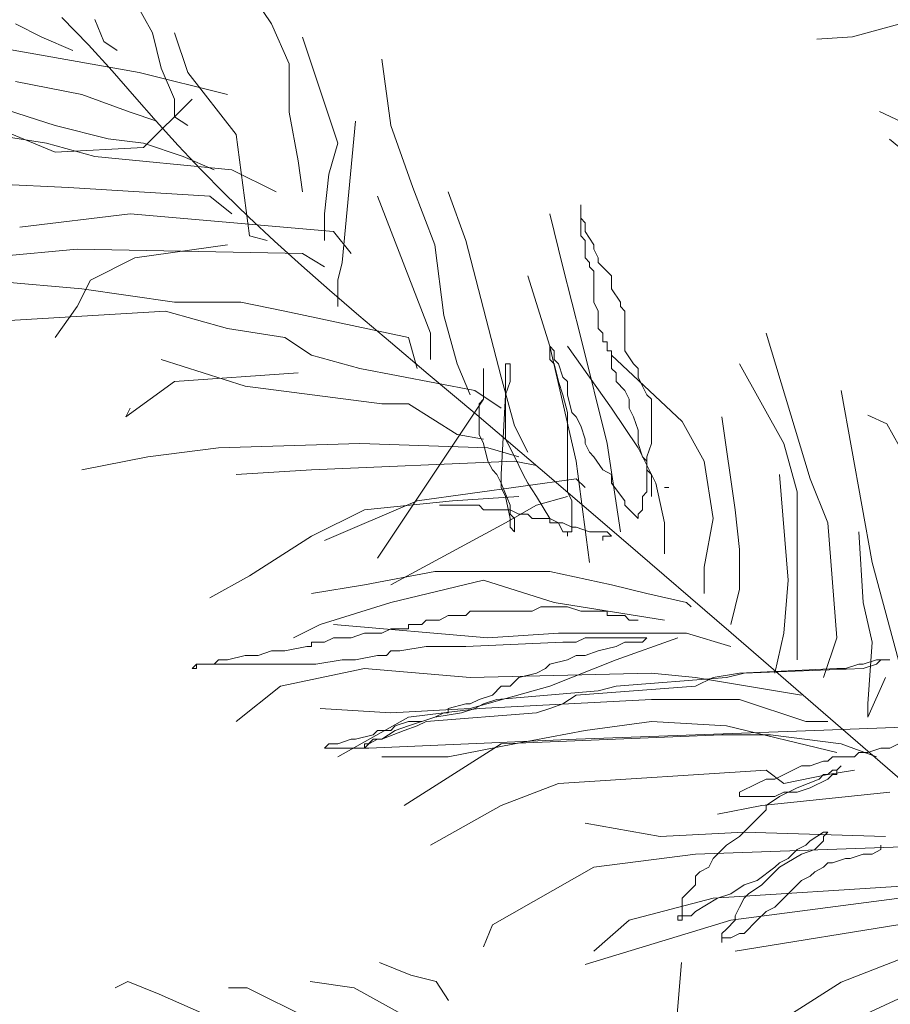
# Model space of a CAD drawing. Units: millimetres. Extents: x 595116 to 630915, y 909473 to 920225.
# Tile 60 of 134: x 629595.727 to 629600.769, y 919295.882 to 919301.582. Entities that reach past the tile are written whole.
import ezdxf

# ---------------------------------------------------------------- set-up
doc = ezdxf.new("R2010")
doc.units = ezdxf.units.MM
doc.layers.add('Dimension', color=3, linetype='Continuous', lineweight=18)
doc.layers.add('L-PLNT', color=85, linetype='Continuous', lineweight=13)
doc.styles.get("Standard").update_dxf_attribs({"font": 'arial.ttf'})
doc.dimstyles.new('ISO-25', dxfattribs={"dimtxt": 9, "dimasz": 6, "dimexe": 1.25, "dimexo": 0.625, "dimtad": 1, "dimlunit": 4, "dimtxsty": 'Standard', "dimcen": 2.5, "dimadec": 0, "dimazin": 0, "dimtfac": 1, "dimtmove": 0, "dimatfit": 3, "dimfxl": 1, "dimarcsym": 0})

# ---------------------------------------------------------------- blocks, each defined once
blk = doc.blocks.new('A$C4FB75ABC')
for p, q in [((1.2153, 3.9442), (1.2902, 3.808)), ((1.3924, 3.9442), (1.4742, 3.8217)), ((1.1917, 3.7897), (1.1506, 3.8319)), ((1.2017, 3.8285), (1.2153, 3.7944)), ((2.4664, 3.8281), (2.3706, 3.8017)), ((1.079, 3.8217), (1.1199, 3.8012)), ((1.4742, 3.8217), (1.5014, 3.7604)), ((1.1199, 3.8012), (1.1676, 3.7808)), ((1.2902, 3.808), (1.3039, 3.7536)), ((1.3243, 3.808), (1.3447, 3.7467)), ((1.5219, 3.8012), (1.5764, 3.6378)), ((2.3706, 3.8017), (2.3152, 3.798)), ((1.0382, 3.7876), (1.2698, 3.7467)), ((1.2284, 3.7492), (1.1917, 3.7897)), ((1.2153, 3.7944), (1.2357, 3.7808)), ((1.6445, 3.7672), (1.6581, 3.665)), ((1.3039, 3.7536), (1.3243, 3.7059)), ((1.5014, 3.7604), (1.5014, 3.6855)), ((1.2625, 3.7099), (1.2284, 3.7492)), ((1.2698, 3.7467), (1.4061, 3.7127)), ((1.3447, 3.7467), (1.4197, 3.6514)), ((1.079, 3.7331), (1.1812, 3.7127)), ((0.97, 3.7195), (1.1403, 3.665)), ((1.1812, 3.7127), (1.2562, 3.6855)), ((1.2959, 3.6716), (1.2625, 3.7099)), ((1.3515, 3.7059), (1.2766, 3.631)), ((1.3243, 3.7059), (1.3243, 3.6787)), ((1.2562, 3.6855), (1.297, 3.6718)), ((1.3243, 3.6787), (1.3447, 3.665)), ((1.5014, 3.6855), (1.5151, 3.6106)), ((2.4899, 3.6502), (2.4119, 3.6869)), ((0.9155, 3.6718), (1.1267, 3.6378)), ((1.1403, 3.6242), (1.0245, 3.6718)), ((1.1403, 3.665), (1.2221, 3.6446)), ((1.3299, 3.6341), (1.2959, 3.6716)), ((1.6036, 3.6718), (1.5832, 3.4539)), ((1.6581, 3.665), (1.6922, 3.5697)), ((1.2221, 3.6446), (1.2766, 3.6378)), ((1.4197, 3.6514), (1.4401, 3.4948)), ((1.1267, 3.6378), (1.2017, 3.6174)), ((1.2766, 3.631), (1.1403, 3.6242)), ((1.2766, 3.6378), (1.3379, 3.6174)), ((1.365, 3.5971), (1.3299, 3.6341)), ((1.5764, 3.6378), (1.5627, 3.5901)), ((2.4618, 3.6157), (2.4274, 3.6439)), ((1.2017, 3.6174), (1.4129, 3.5969)), ((1.3379, 3.6174), (1.3856, 3.5969)), ((1.5151, 3.6106), (1.5219, 3.5629)), ((1.4014, 3.5604), (1.365, 3.5971)), ((1.4129, 3.5969), (1.481, 3.5629)), ((1.5627, 3.5901), (1.5559, 3.5288)), ((1.0177, 3.5765), (1.1608, 3.5697)), ((1.1608, 3.5697), (1.3788, 3.5561)), ((1.6922, 3.5697), (1.7263, 3.4812)), ((1.3788, 3.5561), (1.4129, 3.5288)), ((1.4393, 3.5237), (1.4014, 3.5604)), ((1.6377, 3.5561), (1.7194, 3.345)), ((1.7467, 3.5629), (1.7739, 3.488)), ((1.9511, 3.4948), (1.9511, 3.5425)), ((1.9511, 3.5425), (1.9511, 3.522)), ((1.0858, 3.5084), (1.2562, 3.5288)), ((1.2562, 3.5288), (1.5696, 3.5016)), ((1.4788, 3.4868), (1.4393, 3.5237)), ((1.5559, 3.5288), (1.5559, 3.488)), ((1.9034, 3.5288), (1.9238, 3.4471)), ((1.9511, 3.522), (1.9579, 3.5152)), ((1.9579, 3.5152), (1.9579, 3.5016)), ((1.4401, 3.4948), (1.4674, 3.488)), ((1.5696, 3.5016), (1.5968, 3.4676)), ((1.9579, 3.488), (1.9511, 3.4948)), ((1.9579, 3.5016), (1.9715, 3.4812)), ((1.4061, 3.4812), (1.263, 3.4608)), ((1.5201, 3.4494), (1.4788, 3.4868)), ((1.7263, 3.4812), (1.7399, 3.3722)), ((1.7739, 3.488), (1.8285, 3.2769)), ((1.9579, 3.4608), (1.9579, 3.488)), ((1.9715, 3.4812), (1.9715, 3.4744)), ((1.0245, 3.4608), (1.1744, 3.4744)), ((1.1744, 3.4744), (1.5219, 3.4676)), ((1.5219, 3.4676), (1.5559, 3.4471)), ((1.9715, 3.4744), (1.9783, 3.4608)), ((1.263, 3.4608), (1.1949, 3.4267)), ((1.5633, 3.4112), (1.5201, 3.4494)), ((1.5832, 3.4539), (1.5764, 3.4267)), ((1.9238, 3.4471), (1.9511, 3.3382)), ((1.9647, 3.4539), (1.9579, 3.4608)), ((1.9647, 3.4471), (1.9647, 3.4539)), ((1.9715, 3.4403), (1.9647, 3.4471)), ((1.9783, 3.4608), (1.9783, 3.4539)), ((1.9783, 3.4539), (1.9988, 3.4335)), ((1.8693, 3.4335), (1.9034, 3.3246)), ((1.9715, 3.3927), (1.9715, 3.4403)), ((1.9988, 3.4335), (1.9988, 3.4131)), ((1.0245, 3.4267), (1.1812, 3.4131)), ((1.1949, 3.4267), (1.1744, 3.3858)), ((1.5764, 3.4267), (1.5764, 3.3858)), ((1.1812, 3.4131), (1.3243, 3.3927)), ((1.6088, 3.3721), (1.5633, 3.4112)), ((1.9988, 3.4131), (2.0124, 3.3927)), ((1.3243, 3.3927), (1.4265, 3.3927)), ((1.4265, 3.3927), (1.4946, 3.379)), ((1.9783, 3.379), (1.9715, 3.3927)), ((2.0124, 3.3927), (2.0124, 3.3858)), ((0.9768, 3.3586), (1.3107, 3.379)), ((1.1744, 3.3858), (1.1403, 3.3382)), ((1.3107, 3.379), (1.4061, 3.3518)), ((1.4946, 3.379), (1.6854, 3.3382)), ((1.6577, 3.3307), (1.6088, 3.3721)), ((1.7399, 3.3722), (1.7603, 3.2973)), ((1.9783, 3.3518), (1.9783, 3.379)), ((2.0124, 3.3858), (2.0192, 3.379)), ((2.0192, 3.379), (2.0192, 3.3178)), ((1.4061, 3.3518), (1.4946, 3.3382)), ((1.7194, 3.345), (1.7194, 3.3041)), ((1.9851, 3.345), (1.9783, 3.3518)), ((1.9851, 3.3314), (1.9851, 3.345)), ((2.2372, 3.345), (2.3054, 3.1203)), ((1.4946, 3.3382), (1.5355, 3.3109)), ((1.7159, 3.2817), (1.6577, 3.3307)), ((1.6854, 3.3382), (1.699, 3.2905)), ((1.9511, 3.3382), (1.992, 3.1748)), ((1.992, 3.3314), (1.9851, 3.3314)), ((1.992, 3.3178), (1.992, 3.3314)), ((1.5355, 3.3109), (1.6104, 3.2905)), ((1.9102, 3.3178), (1.9034, 3.3246)), ((1.9034, 3.3246), (1.9034, 3.3041)), ((1.9034, 3.3246), (1.9443, 3.1475)), ((1.9102, 3.3041), (1.9102, 3.3178)), ((1.9306, 3.3246), (1.9988, 3.2292)), ((1.9988, 3.3178), (1.992, 3.3178)), ((1.9988, 3.2905), (1.9988, 3.3178)), ((1.9988, 3.3109), (2.1078, 3.2088)), ((2.0192, 3.3178), (2.0328, 3.2973)), ((1.3039, 3.3041), (1.4333, 3.2633)), ((1.7603, 3.2973), (1.7808, 3.2497)), ((1.8421, 3.2973), (1.8353, 3.2973)), ((1.8353, 3.2973), (1.8353, 3.2497)), ((1.8421, 3.2701), (1.8421, 3.2973)), ((1.9034, 3.3041), (1.9102, 3.2973)), ((1.917, 3.2973), (1.9102, 3.3041)), ((1.9102, 3.2973), (1.917, 3.2701)), ((1.9238, 3.2769), (1.917, 3.2973)), ((2.0328, 3.2973), (2.0396, 3.2905)), ((2.1963, 3.2973), (2.2645, 3.1748)), ((1.5151, 3.2837), (1.3243, 3.2701)), ((1.6104, 3.2905), (1.7876, 3.2565)), ((1.7906, 3.2188), (1.7159, 3.2817)), ((1.8012, 3.2429), (1.8012, 3.2905)), ((1.8012, 3.2905), (1.8012, 3.2429)), ((2.0056, 3.2837), (1.9988, 3.2905)), ((2.0056, 3.2701), (2.0056, 3.2837)), ((2.0396, 3.2905), (2.0396, 3.2769)), ((1.3243, 3.2701), (1.2494, 3.2156)), ((1.8285, 3.2769), (1.8489, 3.202)), ((1.8353, 3.2497), (1.8421, 3.2701)), ((1.917, 3.2701), (1.9238, 3.2497)), ((1.9306, 3.2701), (1.9238, 3.2769)), ((1.9306, 3.2497), (1.9306, 3.2701)), ((2.0192, 3.2565), (2.0056, 3.2701)), ((2.0396, 3.2769), (2.0465, 3.2633)), ((1.4333, 3.2633), (1.6445, 3.236)), ((1.7876, 3.2565), (1.8285, 3.2292)), ((1.8353, 3.2497), (1.8285, 3.1271)), ((1.8353, 3.1816), (1.8353, 3.2497)), ((1.9238, 3.2497), (1.9306, 3.2224)), ((1.9375, 3.2224), (1.9306, 3.2497)), ((2.026, 3.2429), (2.0192, 3.2565)), ((2.0465, 3.2633), (2.0533, 3.2497)), ((2.0533, 3.2497), (2.0601, 3.2429)), ((2.353, 3.2565), (2.4007, 2.9909)), ((1.8012, 3.2429), (1.6377, 2.9977)), ((1.6445, 3.236), (1.6854, 3.236)), ((1.6854, 3.236), (1.7603, 3.1884)), ((1.7944, 3.236), (1.8012, 3.2429)), ((1.7944, 3.1884), (1.7944, 3.236)), ((2.026, 3.2292), (2.026, 3.2429)), ((2.0601, 3.2429), (2.0601, 3.1748)), ((1.2494, 3.2156), (1.2562, 3.2292)), ((1.9306, 3.2224), (1.9306, 3.0999)), ((1.9443, 3.2156), (1.9375, 3.2224)), ((1.9988, 3.2292), (2.0396, 3.1679)), ((2.0328, 3.2156), (2.026, 3.2292)), ((1.8887, 3.1355), (1.7906, 3.2188)), ((1.9511, 3.202), (1.9443, 3.2156)), ((2.0396, 3.1952), (2.0328, 3.2156)), ((2.1078, 3.2088), (2.1418, 3.1475)), ((2.1691, 3.2156), (2.1895, 3.0726)), ((2.4234, 3.2048), (2.3941, 3.2186)), ((2.4914, 3.0833), (2.4234, 3.2048)), ((1.8489, 3.202), (1.8693, 3.1611)), ((1.9579, 3.1816), (1.9511, 3.202)), ((2.0396, 3.1748), (2.0396, 3.1952)), ((1.3924, 3.1679), (1.6104, 3.1748)), ((1.6104, 3.1748), (1.808, 3.1679)), ((1.7603, 3.1884), (1.8012, 3.1816)), ((1.8012, 3.1748), (1.7944, 3.1884)), ((1.808, 3.1475), (1.8012, 3.1748)), ((1.8421, 3.1679), (1.8353, 3.1816)), ((1.9579, 3.1748), (1.9579, 3.1816)), ((1.9647, 3.1611), (1.9579, 3.1748)), ((1.992, 3.1748), (2.0124, 3.0386)), ((2.0465, 3.1543), (2.0396, 3.1748)), ((2.0601, 3.1748), (2.0533, 3.1543)), ((2.2645, 3.1748), (2.2849, 3.0999)), ((1.2834, 3.1543), (1.3924, 3.1679)), ((1.808, 3.1679), (1.8557, 3.1543)), ((1.8557, 3.1407), (1.8421, 3.1679)), ((1.9715, 3.1543), (1.9647, 3.1611)), ((2.0396, 3.1679), (2.0669, 3.1135)), ((1.1812, 3.1339), (1.2834, 3.1543)), ((1.5355, 3.1339), (1.8489, 3.1475)), ((1.8148, 3.1339), (1.808, 3.1475)), ((1.8489, 3.1475), (1.883, 3.1407)), ((1.9443, 3.1475), (1.9647, 2.9909)), ((1.9851, 3.1339), (1.9715, 3.1543)), ((2.0533, 3.1475), (2.0465, 3.1543)), ((2.0533, 3.1543), (2.0533, 3.0999)), ((2.0533, 3.1339), (2.0533, 3.1475)), ((2.1418, 3.1475), (2.1555, 3.059)), ((1.4197, 3.1271), (1.5355, 3.1339)), ((1.8216, 3.1271), (1.8148, 3.1339)), ((1.8625, 3.1271), (1.8557, 3.1407)), ((2.0174, 3.0255), (1.8887, 3.1355)), ((1.9988, 3.1271), (1.9851, 3.1339)), ((2.0601, 3.1271), (2.0533, 3.1339)), ((1.699, 3.0862), (1.9443, 3.1203)), ((1.8285, 3.1135), (1.8216, 3.1271)), ((1.8285, 3.1271), (1.8285, 3.1067)), ((1.8421, 3.0794), (1.8285, 3.1135)), ((1.8693, 3.1135), (1.8625, 3.1271)), ((1.883, 3.093), (1.8693, 3.1135)), ((1.9443, 3.1203), (1.9579, 3.1067)), ((1.9988, 3.1135), (1.9988, 3.1271)), ((2.0192, 3.0862), (1.9988, 3.1135)), ((2.0601, 3.093), (2.0601, 3.1271)), ((2.0669, 3.1135), (2.0805, 3.0522)), ((2.2577, 3.1271), (2.2713, 2.9637)), ((2.3054, 3.1203), (2.3326, 3.0522)), ((1.8285, 3.1067), (1.8353, 3.093)), ((1.9306, 3.0999), (1.9375, 3.0862)), ((2.0533, 3.0999), (2.0465, 3.093)), ((2.0873, 3.1067), (2.0805, 3.1067)), ((2.2849, 3.0999), (2.2849, 2.9024)), ((1.5559, 3.0249), (1.699, 3.0862)), ((1.7535, 3.0862), (1.6173, 3.0726)), ((1.8557, 3.093), (1.7535, 3.0862)), ((1.8353, 3.093), (1.8421, 3.059)), ((1.9034, 3.059), (1.883, 3.093)), ((1.883, 3.0794), (1.9306, 3.093)), ((1.9375, 3.0862), (1.9375, 3.0386)), ((2.0192, 3.0794), (2.0192, 3.0862)), ((2.0465, 3.093), (2.0465, 3.0726)), ((1.6173, 3.0726), (1.5355, 3.0318)), ((1.7331, 3.0794), (1.7944, 3.0794)), ((1.7944, 3.0794), (1.8012, 3.0726)), ((1.8012, 3.0726), (1.8421, 3.0726)), ((1.8353, 3.0522), (1.883, 3.0794)), ((1.8421, 3.0658), (1.8421, 3.0794)), ((1.8421, 3.0726), (1.8557, 3.0658)), ((2.0396, 3.059), (2.0192, 3.0794)), ((2.0465, 3.0726), (2.0396, 3.0658)), ((2.1895, 3.0726), (2.1963, 3.0113)), ((1.8489, 3.059), (1.8421, 3.0658)), ((1.8421, 3.059), (1.8421, 3.0454)), ((1.8489, 3.0386), (1.8489, 3.059)), ((1.8557, 3.0658), (1.8693, 3.0658)), ((1.8693, 3.0658), (1.8761, 3.059)), ((1.8761, 3.059), (1.9034, 3.059)), ((1.917, 3.0522), (1.9034, 3.059)), ((1.9034, 3.059), (1.9034, 3.0522)), ((2.0396, 3.0658), (2.0396, 3.059)), ((2.1555, 3.059), (2.1418, 2.9841)), ((1.6581, 2.9569), (1.8353, 3.0522)), ((1.8421, 3.0454), (1.8489, 3.0386)), ((1.9034, 3.0522), (1.9238, 3.0522)), ((1.9238, 3.0386), (1.917, 3.0522)), ((1.9238, 3.0522), (1.9375, 3.0454)), ((1.9306, 3.0386), (1.9238, 3.0386)), ((1.9375, 3.0386), (1.9306, 3.0386)), ((1.9306, 3.0386), (1.9306, 3.0318)), ((1.9306, 3.0318), (1.9306, 3.0386)), ((1.9375, 3.0454), (1.9443, 3.0454)), ((1.9443, 3.0454), (1.9647, 3.0386)), ((1.9647, 3.0386), (1.992, 3.0386)), ((1.992, 3.0386), (1.9988, 3.0318)), ((2.0805, 3.0522), (2.0805, 3.0045)), ((2.3326, 3.0522), (2.3462, 2.8751)), ((2.3803, 3.0386), (2.3871, 2.9296)), ((1.5355, 3.0318), (1.4401, 2.9705)), ((1.9988, 3.0318), (1.9851, 3.0318)), ((1.9851, 3.0318), (1.9851, 3.0249)), ((2.1835, 2.8826), (2.0174, 3.0255)), ((2.1963, 3.0113), (2.1963, 2.95)), ((1.6173, 2.9569), (1.7263, 2.9773)), ((1.7263, 2.9773), (1.9034, 2.9773)), ((1.9034, 2.9773), (1.9988, 2.9569)), ((2.1418, 2.9841), (2.1418, 2.9432)), ((2.4007, 2.9909), (2.4484, 2.8139)), ((1.4401, 2.9705), (1.3788, 2.9364)), ((1.8012, 2.9637), (1.6581, 2.9296)), ((1.9102, 2.9296), (1.8012, 2.9637)), ((2.2713, 2.9637), (2.2645, 2.882)), ((1.5355, 2.9432), (1.6173, 2.9569)), ((1.9988, 2.9569), (2.0533, 2.9432)), ((2.1963, 2.95), (2.1827, 2.8956)), ((2.0533, 2.9432), (2.1146, 2.9296)), ((1.6581, 2.9296), (1.5491, 2.8956)), ((1.7808, 2.916), (1.7739, 2.9092)), ((1.8761, 2.916), (1.7808, 2.916)), ((1.8898, 2.9228), (1.8761, 2.916)), ((1.9306, 2.9228), (1.8898, 2.9228)), ((2.0805, 2.9024), (1.9102, 2.9296)), ((1.9511, 2.916), (1.9306, 2.9228)), ((1.992, 2.916), (1.9511, 2.916)), ((1.992, 2.9092), (1.992, 2.916)), ((2.1146, 2.9296), (2.1214, 2.9228)), ((2.3871, 2.9296), (2.4007, 2.8683)), ((1.7126, 2.9024), (1.7058, 2.8956)), ((1.7331, 2.9024), (1.7126, 2.9024)), ((1.7467, 2.9092), (1.7331, 2.9024)), ((1.7739, 2.9092), (1.7467, 2.9092)), ((2.0192, 2.9092), (1.992, 2.9092)), ((2.026, 2.9024), (2.0192, 2.9092)), ((2.0396, 2.9024), (2.026, 2.9024)), ((2.2849, 2.9024), (2.2849, 2.8411)), ((1.5491, 2.8956), (1.5082, 2.8751)), ((1.5696, 2.8956), (1.808, 2.8751)), ((1.6581, 2.8888), (1.6445, 2.882)), ((1.6854, 2.8888), (1.6581, 2.8888)), ((1.6854, 2.8956), (1.6854, 2.8888)), ((1.7058, 2.8956), (1.6854, 2.8956)), ((1.5696, 2.8751), (1.5559, 2.8683)), ((1.5968, 2.8751), (1.5696, 2.8751)), ((1.6173, 2.882), (1.5968, 2.8751)), ((1.6445, 2.882), (1.6173, 2.882)), ((1.808, 2.8751), (1.917, 2.882)), ((1.917, 2.882), (2.1146, 2.882)), ((1.9443, 2.8683), (1.9579, 2.8751)), ((1.9579, 2.8751), (2.0533, 2.8751)), ((2.101, 2.8751), (2.0056, 2.8411)), ((2.0533, 2.8751), (2.0465, 2.8683)), ((2.1146, 2.882), (2.1827, 2.8615)), ((2.3943, 2.7002), (2.1835, 2.8826)), ((2.2645, 2.882), (2.2508, 2.8207)), ((2.3462, 2.8751), (2.3258, 2.8139)), ((1.5287, 2.8615), (1.4946, 2.8547)), ((1.5355, 2.8615), (1.5287, 2.8615)), ((1.5559, 2.8683), (1.5355, 2.8683)), ((1.5355, 2.8683), (1.5355, 2.8615)), ((1.6718, 2.8547), (1.7126, 2.8615)), ((1.7126, 2.8615), (1.7739, 2.8615)), ((1.7739, 2.8615), (1.9238, 2.8683)), ((1.9238, 2.8683), (1.9443, 2.8683)), ((2.0056, 2.8615), (1.9783, 2.8547)), ((2.0192, 2.8683), (2.0056, 2.8615)), ((2.0465, 2.8683), (2.0192, 2.8683)), ((2.4007, 2.8683), (2.3939, 2.773)), ((1.3924, 2.8411), (1.3856, 2.8343)), ((1.4061, 2.8411), (1.3924, 2.8411)), ((1.4333, 2.8479), (1.4061, 2.8411)), ((1.4537, 2.8479), (1.4333, 2.8479)), ((1.4742, 2.8547), (1.4537, 2.8479)), ((1.4946, 2.8547), (1.4742, 2.8547)), ((1.5423, 2.8343), (1.5832, 2.8411)), ((1.5832, 2.8411), (1.6036, 2.8411)), ((1.6036, 2.8411), (1.6377, 2.8479)), ((1.6377, 2.8479), (1.6513, 2.8479)), ((1.6513, 2.8479), (1.6581, 2.8547)), ((1.6581, 2.8547), (1.6718, 2.8547)), ((1.9306, 2.8411), (1.9034, 2.8343)), ((2.0056, 2.8411), (1.9034, 2.8002)), ((1.9443, 2.8479), (1.9306, 2.8411)), ((1.9579, 2.8479), (1.9443, 2.8479)), ((1.9783, 2.8547), (1.9579, 2.8479)), ((2.3871, 2.8343), (2.4075, 2.8411)), ((2.4075, 2.8411), (2.428, 2.8411)), ((2.4144, 2.8411), (2.4075, 2.8343)), ((2.428, 2.8411), (2.4144, 2.8411)), ((1.3515, 2.8275), (1.3584, 2.8343)), ((1.3584, 2.8275), (1.3515, 2.8275)), ((1.3856, 2.8343), (1.3584, 2.8343)), ((1.3584, 2.8343), (1.3584, 2.8275)), ((1.3584, 2.8343), (1.5423, 2.8343)), ((1.4878, 2.8002), (1.6173, 2.8275)), ((1.6173, 2.8275), (1.7808, 2.8139)), ((1.8966, 2.8275), (1.883, 2.8207)), ((1.9034, 2.8343), (1.8966, 2.8275)), ((2.1963, 2.8207), (2.3462, 2.8275)), ((2.3871, 2.8275), (2.2032, 2.8207)), ((2.3462, 2.8275), (2.3599, 2.8275)), ((2.3599, 2.8275), (2.3803, 2.8343)), ((2.3803, 2.8343), (2.3871, 2.8343)), ((2.4075, 2.8343), (2.3871, 2.8275)), ((1.7808, 2.8139), (2.0601, 2.8207)), ((1.8557, 2.8139), (1.8421, 2.8002)), ((1.883, 2.8207), (1.8557, 2.8139)), ((2.1759, 2.8139), (2.0056, 2.8002)), ((2.0601, 2.8207), (2.1282, 2.8139)), ((2.1282, 2.8002), (2.1555, 2.8139)), ((2.1282, 2.8139), (2.2917, 2.7866)), ((2.1555, 2.8139), (2.1963, 2.8207)), ((2.2032, 2.8207), (2.1759, 2.8139)), ((2.3939, 2.7526), (2.4212, 2.8139)), ((1.4197, 2.7458), (1.4878, 2.8002)), ((1.9034, 2.8002), (1.7808, 2.7662)), ((1.8285, 2.8002), (1.8148, 2.7866)), ((1.8421, 2.8002), (1.8285, 2.8002)), ((1.9443, 2.7866), (2.1282, 2.8002)), ((2.0056, 2.8002), (1.9783, 2.7934)), ((1.7944, 2.7798), (1.7808, 2.773)), ((1.8148, 2.7866), (1.7944, 2.7798)), ((1.7944, 2.7662), (2.0601, 2.7798)), ((1.8216, 2.7798), (1.8012, 2.773)), ((1.9783, 2.7934), (1.8216, 2.7798)), ((1.9238, 2.773), (1.9443, 2.7866)), ((2.0601, 2.7798), (2.1078, 2.7798)), ((2.1078, 2.7798), (2.1963, 2.7798)), ((2.1963, 2.7798), (2.2985, 2.7458)), ((1.6581, 2.7594), (1.5491, 2.7662)), ((1.7808, 2.7662), (1.6581, 2.7594)), ((1.6854, 2.7526), (1.7944, 2.7662)), ((1.7739, 2.773), (1.7467, 2.7662)), ((1.7467, 2.7662), (1.7467, 2.7594)), ((1.7876, 2.7662), (1.7671, 2.7594)), ((1.7808, 2.773), (1.7739, 2.773)), ((1.8012, 2.773), (1.7876, 2.7662)), ((1.883, 2.7594), (1.9034, 2.7662)), ((1.9034, 2.7662), (1.9238, 2.773)), ((2.3939, 2.773), (2.3939, 2.7526)), ((1.5764, 2.6913), (1.6854, 2.7526)), ((1.7263, 2.7526), (1.6854, 2.739)), ((1.7263, 2.7526), (1.7058, 2.7458)), ((1.7126, 2.7458), (1.883, 2.7594)), ((1.7399, 2.7594), (1.7263, 2.7526)), ((1.7671, 2.7594), (1.7263, 2.7526)), ((1.7467, 2.7594), (1.7399, 2.7594)), ((1.6649, 2.739), (1.6581, 2.7321)), ((1.6854, 2.7458), (1.6649, 2.739)), ((1.6854, 2.739), (1.6649, 2.7321)), ((1.6786, 2.7321), (1.699, 2.739)), ((1.7058, 2.7458), (1.6854, 2.7458)), ((1.699, 2.739), (1.7126, 2.7458)), ((2.0601, 2.7458), (1.9579, 2.7321)), ((2.1759, 2.739), (2.0601, 2.7458)), ((2.3462, 2.6981), (2.1759, 2.739)), ((2.2985, 2.7458), (2.3326, 2.7458)), ((2.3122, 2.7321), (2.4961, 2.739)), ((1.5968, 2.7185), (1.5764, 2.7117)), ((1.6036, 2.7185), (1.5968, 2.7185)), ((1.6309, 2.7253), (1.6036, 2.7185)), ((1.6309, 2.7185), (1.6173, 2.7049)), ((1.6241, 2.7117), (1.6377, 2.7185)), ((1.6241, 2.7049), (1.9443, 2.7185)), ((1.6377, 2.7321), (1.6309, 2.7253)), ((1.6445, 2.7185), (1.6309, 2.7185)), ((1.6581, 2.7321), (1.6377, 2.7321)), ((1.6377, 2.7185), (1.6445, 2.7185)), ((1.6649, 2.7321), (1.6445, 2.7185)), ((1.6445, 2.7185), (1.6786, 2.7321)), ((1.8285, 2.7117), (2.1691, 2.7253)), ((1.9579, 2.7321), (1.8489, 2.7117)), ((1.9443, 2.7185), (2.1282, 2.7253)), ((2.1282, 2.7253), (2.3122, 2.7321)), ((2.1691, 2.7253), (2.244, 2.7253)), ((2.244, 2.7253), (2.353, 2.7117)), ((2.4552, 2.7185), (2.428, 2.7049)), ((1.5627, 2.7117), (1.5559, 2.7049)), ((1.5559, 2.7049), (1.6241, 2.7049)), ((1.5764, 2.7117), (1.5627, 2.7117)), ((1.6173, 2.7049), (1.6173, 2.7117)), ((1.6173, 2.7117), (1.6241, 2.7117)), ((1.6786, 2.6164), (1.8285, 2.7117)), ((1.8489, 2.7117), (1.7467, 2.6913)), ((2.353, 2.7117), (2.4075, 2.6913)), ((2.4144, 2.7049), (2.3939, 2.6981)), ((2.428, 2.7049), (2.4144, 2.7049)), ((1.7467, 2.6913), (1.6445, 2.6913)), ((2.3394, 2.6913), (2.3326, 2.6845)), ((2.3735, 2.6913), (2.3394, 2.6913)), ((2.3803, 2.6981), (2.3735, 2.6913)), ((2.3939, 2.6981), (2.3803, 2.6981)), ((2.6566, 2.472), (2.3943, 2.7002)), ((2.2917, 2.6777), (2.2508, 2.6572)), ((2.3054, 2.6777), (2.2917, 2.6777)), ((2.3258, 2.6845), (2.3054, 2.6777)), ((2.3326, 2.6845), (2.3258, 2.6845)), ((2.3462, 2.6709), (2.353, 2.6777)), ((2.353, 2.6777), (2.3462, 2.6709)), ((1.917, 2.6504), (2.2372, 2.6709)), ((2.2372, 2.6709), (2.2645, 2.6504)), ((2.2645, 2.6504), (2.3326, 2.664)), ((2.3258, 2.664), (2.319, 2.6572)), ((2.3326, 2.664), (2.3258, 2.664)), ((2.3394, 2.6709), (2.3326, 2.664)), ((2.3326, 2.664), (2.3735, 2.6709)), ((2.3326, 2.6572), (2.3394, 2.664)), ((2.3462, 2.6709), (2.3394, 2.6709)), ((2.3394, 2.664), (2.3462, 2.664)), ((2.3462, 2.664), (2.3462, 2.6709)), ((1.8285, 2.6164), (1.917, 2.6504)), ((2.2236, 2.6504), (2.1963, 2.6368)), ((2.2372, 2.6572), (2.2236, 2.6504)), ((2.2508, 2.6572), (2.2372, 2.6572)), ((2.2849, 2.6436), (2.2577, 2.63)), ((2.319, 2.6572), (2.2849, 2.6436)), ((2.2849, 2.6368), (2.3054, 2.6436)), ((2.3054, 2.6436), (2.3326, 2.6572)), ((2.1963, 2.6368), (2.1963, 2.63)), ((2.1963, 2.63), (2.2508, 2.63)), ((2.428, 2.6368), (2.2304, 2.6164)), ((2.2577, 2.63), (2.2372, 2.6164)), ((2.2508, 2.63), (2.2645, 2.6368)), ((2.2645, 2.6368), (2.2849, 2.6368)), ((1.7194, 2.5551), (1.8285, 2.6164)), ((2.2304, 2.6164), (2.1623, 2.6028)), ((2.2372, 2.6164), (2.2372, 2.6096)), ((2.2372, 2.6096), (2.2236, 2.596)), ((2.0737, 2.5687), (1.9579, 2.5891)), ((2.21, 2.5823), (2.1963, 2.5687)), ((2.2236, 2.596), (2.21, 2.5823)), ((2.2032, 2.5755), (2.0737, 2.5687)), ((2.1963, 2.5687), (2.1759, 2.5551)), ((2.4212, 2.5687), (2.2032, 2.5755)), ((2.3054, 2.5619), (2.3258, 2.5755)), ((2.3258, 2.5755), (2.3326, 2.5755)), ((2.3326, 2.5755), (2.3258, 2.5687)), ((2.3258, 2.5687), (2.3258, 2.5619)), ((2.5234, 2.5551), (2.1282, 2.5415)), ((2.1759, 2.5551), (2.1623, 2.5415)), ((2.2849, 2.5483), (2.2985, 2.5551)), ((2.2985, 2.5551), (2.3054, 2.5619)), ((2.3258, 2.5619), (2.3122, 2.5483)), ((2.4144, 2.5483), (2.4144, 2.5551)), ((2.1282, 2.5415), (1.9715, 2.5211)), ((2.1623, 2.5415), (2.1555, 2.5347)), ((2.2917, 2.5415), (2.2577, 2.5211)), ((2.2713, 2.5347), (2.2781, 2.5415)), ((2.2781, 2.5415), (2.2849, 2.5483)), ((2.3122, 2.5483), (2.2917, 2.5415)), ((2.3667, 2.5347), (2.3871, 2.5415)), ((2.3871, 2.5415), (2.4007, 2.5415)), ((2.4007, 2.5415), (2.4144, 2.5483)), ((1.9715, 2.5211), (1.8148, 2.4325)), ((2.1487, 2.5211), (2.135, 2.5142)), ((2.1555, 2.5347), (2.1487, 2.5211)), ((2.2236, 2.5006), (2.2508, 2.5211)), ((2.2577, 2.5211), (2.244, 2.5074)), ((2.2508, 2.5211), (2.2577, 2.5279)), ((2.2577, 2.5279), (2.2713, 2.5347)), ((2.3122, 2.5142), (2.3258, 2.5211)), ((2.3258, 2.5211), (2.3326, 2.5279)), ((2.3326, 2.5279), (2.3394, 2.5279)), ((2.3394, 2.5279), (2.3599, 2.5347)), ((2.3599, 2.5347), (2.3667, 2.5347)), ((2.135, 2.5142), (2.1282, 2.5074)), ((2.1282, 2.5074), (2.1282, 2.4938)), ((2.244, 2.5074), (2.2304, 2.4938)), ((2.2917, 2.5006), (2.3054, 2.5074)), ((2.3054, 2.5074), (2.3122, 2.5142)), ((2.1282, 2.4938), (2.1146, 2.4802)), ((2.5847, 2.5006), (2.1555, 2.4734)), ((2.1827, 2.4802), (2.2032, 2.4938)), ((2.5983, 2.4938), (2.1827, 2.4393)), ((2.2032, 2.4938), (2.2236, 2.5006)), ((2.2304, 2.4938), (2.21, 2.4802)), ((2.2781, 2.487), (2.2917, 2.5006)), ((2.1146, 2.4802), (2.1078, 2.4734)), ((2.1623, 2.4734), (2.1827, 2.4802)), ((2.21, 2.4802), (2.2032, 2.4734)), ((2.2508, 2.4598), (2.2781, 2.487)), ((2.1555, 2.4734), (2.026, 2.4393)), ((2.1078, 2.4734), (2.1078, 2.4461)), ((2.1282, 2.453), (2.1623, 2.4734)), ((2.6528, 2.4666), (2.1895, 2.3917)), ((2.2032, 2.4734), (2.1963, 2.4598)), ((2.1078, 2.4461), (2.101, 2.4461)), ((2.101, 2.4461), (2.101, 2.4393)), ((2.1078, 2.4393), (2.1078, 2.4461)), ((2.1078, 2.4461), (2.1214, 2.4461)), ((2.1214, 2.4461), (2.1282, 2.453)), ((2.1963, 2.4598), (2.1895, 2.4461)), ((2.1895, 2.4461), (2.1895, 2.4393)), ((2.2236, 2.4393), (2.2372, 2.453)), ((2.2372, 2.453), (2.2508, 2.4598)), ((1.8148, 2.4325), (1.8012, 2.3985)), ((2.1827, 2.4393), (1.9579, 2.3712)), ((2.026, 2.4393), (1.9715, 2.3917)), ((2.101, 2.4393), (2.1078, 2.4393)), ((2.1895, 2.4393), (2.1759, 2.4257)), ((2.2032, 2.4189), (2.2236, 2.4393)), ((2.1759, 2.4257), (2.1691, 2.4189)), ((2.1691, 2.4189), (2.1691, 2.4053)), ((2.1827, 2.4121), (2.1963, 2.4189)), ((2.1963, 2.4189), (2.2032, 2.4189)), ((2.1691, 2.4053), (2.1691, 2.4121)), ((2.1691, 2.4121), (2.1827, 2.4121)), ((2.353, 2.344), (2.4757, 2.3917)), ((1.6891, 2.3546), (1.6405, 2.3741)), ((2.1065, 2.3741), (2.087, 2.1315)), ((1.7279, 2.3449), (1.6891, 2.3546)), ((1.2522, 2.3449), (1.2328, 2.3352)), ((1.3008, 2.3255), (1.2522, 2.3449)), ((1.6017, 2.3352), (1.5337, 2.3449)), ((1.7473, 2.3158), (1.7279, 2.3449)), ((2.2781, 2.2963), (2.353, 2.344)), ((1.3881, 2.2867), (1.3008, 2.3255)), ((1.4367, 2.3352), (1.4075, 2.3352)), ((1.5337, 2.2867), (1.4367, 2.3352)), ((1.6891, 2.2867), (1.6017, 2.3352)), ((2.3054, 2.2555), (2.4825, 2.3372))]:
    blk.add_line(p, q)
blk = doc.blocks.new('*D210')
at = {"layer": 'Defpoints', "color": 0, "transparency": 16777216}
for p in [(629586.2273, 919310.1229), (629593.9463, 919310.1229), (629586.2273, 919258.6624)]:
    blk.add_point(p, dxfattribs=at)
at = {"layer": 'Dimension', "color": 0, "lineweight": -2, "transparency": 16777216}
for p, q in [((629593.9463, 919310.1229), (629593.9463, 919449.6901)), ((629586.8523, 919310.1229), (629595.1963, 919310.1229)), ((629593.9463, 919264.6624), (629593.9463, 919304.1229)), ((629586.8523, 919258.6624), (629595.1963, 919258.6624))]:
    blk.add_line(p, q, dxfattribs=at)
at = {"layer": 'Dimension', "color": 0, "transparency": 16777216}
for points in [[(629592.9463, 919304.1229), (629594.9463, 919304.1229), (629593.9463, 919310.1229)], [(629592.9463, 919264.6624), (629594.9463, 919264.6624), (629593.9463, 919258.6624)]]:
    blk.add_solid(points, dxfattribs=at)
at = {"layer": 'Dimension', "color": 0, "transparency": 16777216, "insert": (629588.6617, 919382.9065), "char_height": 9, "attachment_point": 5, "rotation": 90}
blk.add_mtext('CANOPY 4\'-3 1/2" TYP.', dxfattribs=at)
blk = doc.blocks.new('*D216')
at = {"layer": 'Defpoints', "color": 0, "transparency": 16777216}
for p in [(629743.5408, 919411.9276), (629505.0408, 919411.8279), (629743.5408, 918832.3776)]:
    blk.add_point(p, dxfattribs=at)
at = {"layer": 'Dimension', "color": 0, "lineweight": -2, "transparency": 16777216}
for p, q in [((629743.5408, 919411.3026), (629743.5408, 918831.1276)), ((629505.0408, 919411.2029), (629505.0408, 918831.1276)), ((629511.0408, 918832.3776), (629737.5408, 918832.3776))]:
    blk.add_line(p, q, dxfattribs=at)
at = {"layer": 'Dimension', "color": 0, "transparency": 16777216}
for points in [[(629511.0408, 918833.3776), (629511.0408, 918831.3776), (629505.0408, 918832.3776)], [(629737.5408, 918833.3776), (629737.5408, 918831.3776), (629743.5408, 918832.3776)]]:
    blk.add_solid(points, dxfattribs=at)
at = {"layer": 'Dimension', "color": 0, "transparency": 16777216, "insert": (629624.2908, 918837.656), "char_height": 9, "attachment_point": 5}
blk.add_mtext('19\'-10 1/2"', dxfattribs=at)

msp = doc.modelspace()

# ---------------------------------------------------------------- block references
at = {"layer": 'L-PLNT', "xscale": 3.753413438031968, "yscale": 3.753413438031968, "zscale": 3.753413438031968}
msp.add_blockref('A$C4FB75ABC', (629591.6528, 919287.2124), dxfattribs=at)

# ---------------------------------------------------------------- dimensions: what is measured, and where the dimension line sits
at = {"layer": 'Dimension'}
dim = msp.add_linear_dim(base=(629593.9463, 919310.1229), p1=(629586.2273, 919258.6624), p2=(629586.2273, 919310.1229), angle=90, text='CANOPY <> TYP.', dimstyle='ISO-25', override={"dimdec": 1, "dimlfac": 1, "dimrnd": 0, "dimzin": 1, "dimdsep": 46, "dimlunit": 4, "dimfrac": 2}, dxfattribs=at)
dim.commit()
dim.dimension.update_dxf_attribs({"geometry": '*D210', "text_midpoint": (629588.6617, 919382.9065)})
dim = msp.add_linear_dim(base=(629743.5408, 918832.3776), p1=(629505.0408, 919411.8279), p2=(629743.5408, 919411.9276), dimstyle='ISO-25', override={"dimdec": 1, "dimlfac": 1, "dimrnd": 0, "dimzin": 1, "dimdsep": 46, "dimlunit": 4, "dimfrac": 2}, dxfattribs=at)
dim.commit()
dim.dimension.update_dxf_attribs({"geometry": '*D216', "text_midpoint": (629624.2908, 918837.656)})

doc.saveas('drawing.dxf')
